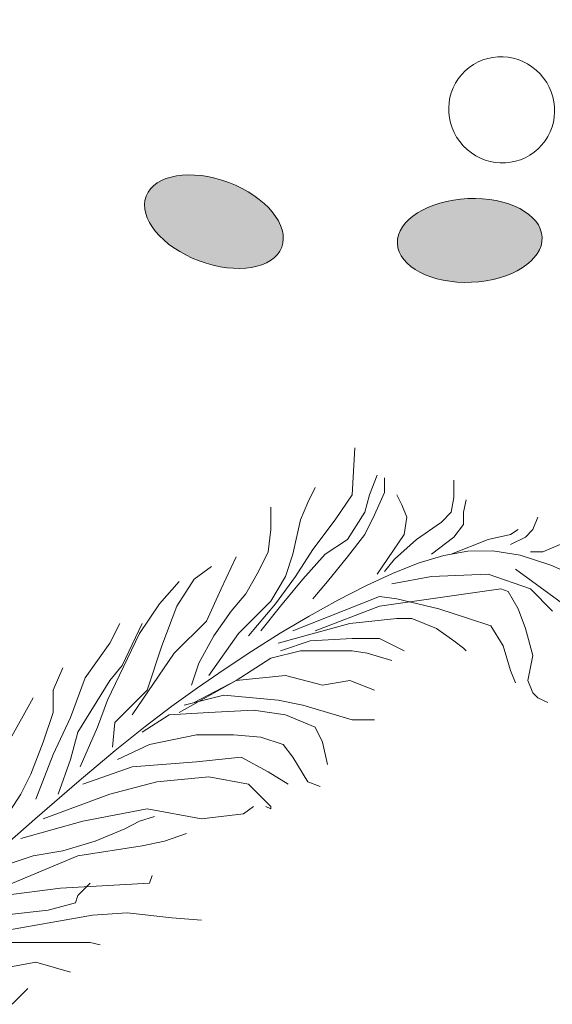
# Model space of a CAD drawing. Units: millimetres. Extents: x 595116 to 630915, y 909473 to 920225.
# Tile 103 of 134: x 629807.854 to 629812.676, y 919172.104 to 919181.018. Entities that reach past the tile are written whole.
import ezdxf

# ---------------------------------------------------------------- set-up
doc = ezdxf.new("R2010")
doc.units = ezdxf.units.MM
doc.layers.add('L-PLNT', color=85, linetype='Continuous', lineweight=13)

# ---------------------------------------------------------------- blocks, each defined once
blk = doc.blocks.new('A$C4FB75ABC')
for p, q in [((4.1608, 3.5609), (4.1668, 3.6742)), ((4.2026, 3.5609), (4.2205, 3.6086)), ((4.2384, 3.5668), (4.2384, 3.6026)), ((4.4054, 3.5549), (4.4054, 3.5967)), ((4.0535, 3.543), (4.0714, 3.5788)), ((4.2145, 3.5132), (4.2384, 3.5668)), ((4.0356, 3.5013), (4.0535, 3.543)), ((4.1191, 3.5013), (4.1608, 3.5609)), ((4.1907, 3.5192), (4.2026, 3.5609)), ((4.2801, 3.537), (4.2682, 3.5609)), ((4.3994, 3.5192), (4.4054, 3.5549)), ((4.4293, 3.5192), (4.4352, 3.549)), ((3.964, 3.4774), (3.964, 3.5311)), ((4.1489, 3.4536), (4.1907, 3.5192)), ((4.2921, 3.5072), (4.2801, 3.537)), ((4.3756, 3.4953), (4.3994, 3.5192)), ((4.4293, 3.4893), (4.4293, 3.5192)), ((4.0177, 3.4178), (4.0356, 3.5013)), ((4.0654, 3.4297), (4.1191, 3.5013)), ((4.1907, 3.4655), (4.2145, 3.5132)), ((4.2861, 3.4655), (4.2921, 3.5072)), ((4.3159, 3.4536), (4.3756, 3.4953)), ((4.5963, 3.4774), (4.6082, 3.5072)), ((3.958, 3.4238), (3.964, 3.4774)), ((4.4054, 3.4595), (4.4293, 3.4893)), ((4.5426, 3.4655), (4.5605, 3.4774)), ((4.5784, 3.4595), (4.5963, 3.4774)), ((4.0952, 3.4178), (4.1489, 3.4536)), ((4.1489, 3.4118), (4.1907, 3.4655)), ((4.2205, 3.3701), (4.2861, 3.4655)), ((4.2622, 3.4059), (4.3159, 3.4536)), ((4.3517, 3.4178), (4.4054, 3.4595)), ((4.3994, 3.4178), (4.4889, 3.4536)), ((4.4889, 3.4536), (4.5426, 3.4655)), ((4.5426, 3.4416), (4.5784, 3.4595)), ((3.9342, 3.3761), (3.958, 3.4238)), ((4.0237, 3.3641), (4.0654, 3.4297)), ((4.3813, 3.4152), (4.4396, 3.4254)), ((4.4396, 3.4254), (4.5001, 3.426)), ((4.5001, 3.426), (4.5657, 3.4153)), ((4.5903, 3.4238), (4.6201, 3.4238)), ((4.6201, 3.4238), (4.6619, 3.4416)), ((3.8447, 3.3343), (3.8805, 3.4118)), ((3.9998, 3.3641), (4.0177, 3.4178)), ((4.0415, 3.3582), (4.0952, 3.4178)), ((4.1012, 3.3522), (4.1489, 3.4118)), ((4.2384, 3.3761), (4.2622, 3.4059)), ((4.2593, 3.3722), (4.322, 3.3969)), ((4.322, 3.3969), (4.3813, 3.4152)), ((4.5657, 3.4153), (4.6395, 3.3917)), ((3.7791, 3.3582), (3.8208, 3.388)), ((3.9044, 3.3224), (3.9342, 3.3761)), ((4.1935, 3.342), (4.2593, 3.3722)), ((4.5545, 3.382), (4.6858, 3.2866)), ((4.6395, 3.3917), (4.7247, 3.3534)), ((3.6956, 3.2986), (3.7433, 3.3522)), ((3.7373, 3.2926), (3.7791, 3.3582)), ((3.964, 3.3045), (3.9998, 3.3641)), ((3.9759, 3.2986), (4.0237, 3.3641)), ((3.9879, 3.2926), (4.0415, 3.3582)), ((4.0654, 3.3105), (4.1012, 3.3522)), ((4.2563, 3.3463), (4.3517, 3.3641)), ((4.3517, 3.3641), (4.4889, 3.3701)), ((4.4889, 3.3701), (4.5903, 3.3343)), ((3.8089, 3.2568), (3.8447, 3.3343)), ((4.1256, 3.3072), (4.1935, 3.342)), ((4.2265, 3.2926), (4.5187, 3.3343)), ((4.5187, 3.3343), (4.5366, 3.3284)), ((4.5366, 3.3284), (4.5605, 3.2866)), ((4.5903, 3.3343), (4.644, 3.2807)), ((3.8686, 3.2807), (3.9044, 3.3224)), ((3.8865, 3.227), (3.964, 3.3045)), ((4.0177, 3.233), (4.2265, 3.3164)), ((4.0565, 3.2687), (4.1256, 3.3072)), ((4.2265, 3.3164), (4.2682, 3.3105)), ((4.2682, 3.3105), (4.3696, 3.2866)), ((3.6479, 3.227), (3.6956, 3.2986)), ((3.7015, 3.1972), (3.7373, 3.2926)), ((3.8268, 3.2211), (3.8686, 3.2807)), ((3.9103, 3.2211), (3.9759, 3.2986)), ((3.9401, 3.233), (3.9879, 3.2926)), ((4.0714, 3.233), (4.2265, 3.2926)), ((4.3696, 3.2866), (4.4412, 3.2628)), ((4.5605, 3.2866), (4.5784, 3.2389)), ((3.7314, 3.1793), (3.8089, 3.2568)), ((3.9871, 3.2274), (4.0565, 3.2687)), ((4.1549, 3.2509), (4.2682, 3.2628)), ((4.2682, 3.2628), (4.304, 3.2628)), ((4.304, 3.2628), (4.3637, 3.2389)), ((4.4412, 3.2628), (4.4949, 3.2449)), ((3.5763, 3.2032), (3.6001, 3.2509)), ((3.6061, 3.1495), (3.6538, 3.2509)), ((3.9819, 3.2032), (4.1549, 3.2509)), ((4.3637, 3.2389), (4.4054, 3.2091)), ((4.4949, 3.2449), (4.5247, 3.1972)), ((4.5784, 3.2389), (4.5963, 3.1734)), ((3.5703, 3.066), (3.6479, 3.227)), ((3.791, 3.1555), (3.8268, 3.2211)), ((3.8149, 3.1257), (3.8865, 3.227)), ((3.9185, 3.1843), (3.9871, 3.2274)), ((3.9879, 3.1853), (4.0594, 3.2091)), ((4.0594, 3.2091), (4.1608, 3.2151)), ((4.1608, 3.2151), (4.2265, 3.2151)), ((4.2265, 3.2151), (4.2861, 3.1853)), ((4.4054, 3.2091), (4.4293, 3.1912)), ((3.5166, 3.1197), (3.5763, 3.2032)), ((3.6658, 3.0899), (3.7015, 3.1972)), ((3.8516, 3.1401), (3.9185, 3.1843)), ((3.964, 3.1674), (4.0356, 3.1853)), ((4.0356, 3.1853), (4.1072, 3.1853)), ((4.1072, 3.1853), (4.1608, 3.1853)), ((4.1608, 3.1853), (4.1966, 3.1793)), ((4.4293, 3.1912), (4.4352, 3.1853)), ((4.5247, 3.1972), (4.5426, 3.1376)), ((3.63, 3.0303), (3.7314, 3.1793)), ((3.8805, 3.1137), (3.964, 3.1674)), ((4.1966, 3.1793), (4.2563, 3.1614)), ((4.5963, 3.1734), (4.5844, 3.1137)), ((3.4391, 3.0899), (3.4629, 3.1436)), ((3.5763, 3.1137), (3.6061, 3.1495)), ((3.7731, 3.1018), (3.791, 3.1555)), ((3.7873, 3.0958), (3.8516, 3.1401)), ((4.5426, 3.1376), (4.5545, 3.1078)), ((3.4808, 3.0243), (3.5166, 3.1197)), ((3.4987, 2.9885), (3.5763, 3.1137)), ((3.7433, 3.0362), (3.8805, 3.1137)), ((3.7791, 3.0601), (3.8805, 3.1137)), ((3.8805, 3.1137), (3.9998, 3.1257)), ((3.9998, 3.1257), (4.0893, 3.1018)), ((4.0893, 3.1018), (4.1549, 3.1137)), ((4.1549, 3.1137), (4.2145, 3.0899)), ((4.5844, 3.1137), (4.5963, 3.0839)), ((3.4391, 3.0362), (3.4391, 3.0899)), ((3.5882, 3.0124), (3.6658, 3.0899)), ((3.7254, 3.0513), (3.7873, 3.0958)), ((3.3317, 2.9647), (3.3914, 3.072)), ((3.5465, 3.0005), (3.5703, 3.066)), ((3.7552, 3.0541), (3.8507, 3.078)), ((3.8507, 3.078), (3.9819, 3.066)), ((3.9819, 3.066), (4.0415, 3.0541)), ((4.5963, 3.0839), (4.6082, 3.072)), ((4.6082, 3.072), (4.6321, 3.0601)), ((3.6611, 3.0024), (3.7254, 3.0513)), ((3.8149, 3.0362), (3.9222, 3.0422)), ((3.9222, 3.0422), (3.9998, 3.0303)), ((4.0415, 3.0541), (4.1608, 3.0184)), ((3.4152, 2.9647), (3.4391, 3.0362)), ((3.4391, 2.9349), (3.4808, 3.0243)), ((3.6538, 2.9885), (3.7194, 3.0303)), ((3.7194, 3.0303), (3.8149, 3.0362)), ((3.9998, 3.0303), (4.0714, 3.0005)), ((4.1608, 3.0184), (4.2145, 3.0184)), ((3.5047, 2.9051), (3.5465, 3.0005)), ((3.5822, 2.9528), (3.5882, 3.0124)), ((3.5886, 2.9442), (3.6611, 3.0024)), ((4.0714, 3.0005), (4.0893, 2.9647)), ((3.4808, 2.923), (3.4987, 2.9885)), ((3.6717, 2.9587), (3.7851, 2.9826)), ((3.7851, 2.9826), (3.8745, 2.9826)), ((3.8745, 2.9826), (3.9401, 2.9766)), ((3.9401, 2.9766), (3.9938, 2.9587)), ((3.3854, 2.8872), (3.4152, 2.9647)), ((3.5942, 2.923), (3.6717, 2.9587)), ((3.9938, 2.9587), (4.0177, 2.9289)), ((4.0893, 2.9647), (4.1012, 2.911)), ((3.3973, 2.8276), (3.4391, 2.9349)), ((3.451, 2.8395), (3.4808, 2.923)), ((3.5019, 2.8714), (3.5886, 2.9442)), ((3.7851, 2.917), (3.8924, 2.9289)), ((3.8924, 2.9289), (3.958, 2.8932)), ((4.0177, 2.9289), (4.0535, 2.8693)), ((3.5107, 2.8633), (3.63, 2.9051)), ((3.63, 2.9051), (3.7851, 2.917)), ((3.3615, 2.8395), (3.3854, 2.8872)), ((3.6896, 2.8693), (3.8149, 2.8812)), ((3.8149, 2.8812), (3.9103, 2.8633)), ((3.958, 2.8932), (4.0058, 2.8633)), ((3.3951, 2.779), (3.5019, 2.8714)), ((3.5763, 2.8395), (3.6896, 2.8693)), ((3.9103, 2.8633), (3.964, 2.8097)), ((4.0535, 2.8693), (4.0833, 2.8574)), ((3.2721, 2.7024), (3.3615, 2.8395)), ((3.4152, 2.7799), (3.5763, 2.8395)), ((3.5107, 2.7739), (3.6658, 2.8037)), ((3.6658, 2.8037), (3.797, 2.7799)), ((3.8984, 2.7918), (3.9222, 2.8097)), ((3.964, 2.8037), (3.9521, 2.8097)), ((3.964, 2.8097), (3.964, 2.8037)), ((3.2623, 2.6619), (3.3951, 2.779)), ((3.6479, 2.7739), (3.6837, 2.7858)), ((3.797, 2.7799), (3.8984, 2.7918)), ((3.3615, 2.7322), (3.5107, 2.7739)), ((3.5405, 2.7262), (3.6121, 2.756)), ((3.6121, 2.756), (3.6479, 2.7739)), ((3.7075, 2.7262), (3.7612, 2.7441)), ((3.4629, 2.7024), (3.5405, 2.7262)), ((3.4987, 2.6904), (3.6538, 2.7143)), ((3.6538, 2.7143), (3.7075, 2.7262)), ((3.2422, 2.5831), (3.4987, 2.6904)), ((3.284, 2.6547), (3.3914, 2.6904)), ((3.3914, 2.6904), (3.4629, 2.7024)), ((3.6717, 2.6249), (3.6777, 2.6428)), ((3.3198, 2.5951), (3.457, 2.6129)), ((3.457, 2.6129), (3.6717, 2.6249)), ((3.4987, 2.5951), (3.5286, 2.6249)), ((3.4928, 2.5772), (3.4987, 2.5951)), ((3.4272, 2.5593), (3.4928, 2.5772)), ((3.1289, 2.4758), (3.5345, 2.5474)), ((3.3198, 2.5474), (3.4272, 2.5593)), ((3.5345, 2.5474), (3.618, 2.5533)), ((3.618, 2.5533), (3.7254, 2.5414)), ((3.7254, 2.5414), (3.797, 2.5354)), ((3.3019, 2.4818), (3.4152, 2.4818)), ((3.4152, 2.4818), (3.5286, 2.4818)), ((3.5286, 2.4818), (3.5524, 2.4758)), ((3.3019, 2.4162), (3.3973, 2.4341)), ((3.3973, 2.4341), (3.4808, 2.4102)), ((3.3403, 2.3324), (3.3784, 2.3706))]:
    blk.add_line(p, q)
blk = doc.blocks.new('A$C77972600')
h = blk.add_hatch(color=256)
edge = h.paths.add_edge_path()
edge.add_ellipse((3.2403, 1.6985), major_axis=(-0.1668, -0.0838), ratio=0.578492, start_angle=0, end_angle=360, ccw=False)
edge = h.paths.add_edge_path()
edge.add_ellipse((4.2796, 1.6084), major_axis=(-0.1206, -0.1425), ratio=0.578492, start_angle=0, end_angle=360, ccw=False)
edge = h.paths.add_edge_path()
edge.add_ellipse((4.7739, 0.881), major_axis=(-0.1747, 0.0657), ratio=0.578492, start_angle=0, end_angle=360, ccw=False)
edge = h.paths.add_edge_path()
edge.add_ellipse((5.4333, 0.8328), major_axis=(-0.1865, -0.008), ratio=0.578492, start_angle=0, end_angle=360, ccw=False)
edge = h.paths.add_edge_path()
edge.add_ellipse((4.6573, 4.2045), major_axis=(-0.1865, -0.008), ratio=0.578492, start_angle=0, end_angle=360, ccw=False)
edge = h.paths.add_edge_path()
edge.add_ellipse((4.556, 3.4032), major_axis=(-0.1865, -0.008), ratio=0.578492, start_angle=0, end_angle=360, ccw=False)
edge = h.paths.add_edge_path()
edge.add_ellipse((4.9297, 3.677), major_axis=(-0.1668, -0.0838), ratio=0.578492, start_angle=0, end_angle=360, ccw=False)
edge = h.paths.add_edge_path()
edge.add_ellipse((3.7756, 2.5742), major_axis=(-0.1206, -0.1425), ratio=0.578492, start_angle=0, end_angle=360, ccw=False)
edge = h.paths.add_edge_path()
edge.add_ellipse((3.1788, 2.8466), major_axis=(-0.1206, -0.1425), ratio=0.578492, start_angle=0, end_angle=360, ccw=False)
edge = h.paths.add_edge_path()
edge.add_ellipse((3.8763, 3.0252), major_axis=(-0.1206, -0.1425), ratio=0.578492, start_angle=0, end_angle=360, ccw=False)
edge = h.paths.add_edge_path()
edge.add_ellipse((2.3609, 1.8217), major_axis=(-0.1865, -0.008), ratio=0.578492, start_angle=0, end_angle=360, ccw=False)
edge = h.paths.add_edge_path()
edge.add_ellipse((3.0627, 1.8578), major_axis=(-0.1865, -0.008), ratio=0.578492, start_angle=0, end_angle=360, ccw=False)
edge = h.paths.add_edge_path()
edge.add_ellipse((2.7605, 2.0535), major_axis=(-0.1865, -0.008), ratio=0.578492, start_angle=0, end_angle=360, ccw=False)
edge = h.paths.add_edge_path()
edge.add_ellipse((2.1439, 3.4246), major_axis=(-0.1668, -0.0838), ratio=0.578492, start_angle=0, end_angle=360, ccw=False)
edge = h.paths.add_edge_path()
edge.add_ellipse((4.2959, 2.0225), major_axis=(-0.1747, 0.0657), ratio=0.578492, start_angle=0, end_angle=360, ccw=False)
edge = h.paths.add_edge_path()
edge.add_ellipse((1.9127, 4.2528), major_axis=(-0.1865, -0.008), ratio=0.578492, start_angle=0, end_angle=360, ccw=False)
edge = h.paths.add_edge_path()
edge.add_ellipse((1.5555, 4.1052), major_axis=(-0.1747, 0.0657), ratio=0.578492, start_angle=0, end_angle=360, ccw=False)
edge = h.paths.add_edge_path()
edge.add_ellipse((0.9962, 4.2695), major_axis=(-0.1865, -0.008), ratio=0.578492, start_angle=0, end_angle=360, ccw=False)
edge = h.paths.add_edge_path()
edge.add_ellipse((1.2179, 3.5926), major_axis=(-0.1747, 0.0657), ratio=0.578492, start_angle=0, end_angle=360, ccw=False)
edge = h.paths.add_edge_path()
edge.add_ellipse((1.6764, 3.6493), major_axis=(-0.1747, 0.0657), ratio=0.578492, start_angle=0, end_angle=360, ccw=False)
edge = h.paths.add_edge_path()
edge.add_ellipse((0.8384, 2.8599), major_axis=(-0.1668, -0.0838), ratio=0.578492, start_angle=0, end_angle=360, ccw=False)
edge = h.paths.add_edge_path()
edge.add_ellipse((0.9659, 2.049), major_axis=(-0.1206, -0.1425), ratio=0.578492, start_angle=0, end_angle=360, ccw=False)
edge = h.paths.add_edge_path()
edge.add_ellipse((1.3147, 2.1383), major_axis=(-0.1206, -0.1425), ratio=0.578492, start_angle=0, end_angle=360, ccw=False)
edge = h.paths.add_edge_path()
edge.add_ellipse((5.4586, 2.9929), major_axis=(-0.1865, -0.008), ratio=0.578492, start_angle=0, end_angle=360, ccw=False)
edge = h.paths.add_edge_path()
edge.add_ellipse((3.4224, 5.3915), major_axis=(-0.1865, -0.008), ratio=0.578492, start_angle=0, end_angle=360, ccw=False)
edge = h.paths.add_edge_path()
edge.add_ellipse((3.7245, 5.1958), major_axis=(-0.1865, -0.008), ratio=0.578492, start_angle=0, end_angle=360, ccw=False)
edge = h.paths.add_edge_path()
edge.add_ellipse((4.5588, 5.4431), major_axis=(-0.1668, -0.0838), ratio=0.578492, start_angle=0, end_angle=360, ccw=False)
edge = h.paths.add_edge_path()
edge.add_ellipse((4.4393, 4.7252), major_axis=(-0.1668, -0.0838), ratio=0.578492, start_angle=0, end_angle=360, ccw=False)
edge = h.paths.add_edge_path()
edge.add_ellipse((4.7087, 5.1006), major_axis=(-0.1668, -0.0838), ratio=0.578492, start_angle=0, end_angle=360, ccw=False)
edge = h.paths.add_edge_path()
edge.add_ellipse((3.7138, 4.6852), major_axis=(-0.1668, -0.0838), ratio=0.578492, start_angle=0, end_angle=360, ccw=False)
blk.add_ellipse((5.5155, 1.1693), major_axis=(-0.0941, 0.1005), ratio=0.985729)
at = {"extrusion": (0, 0, -1)}
blk.add_ellipse((4.7739, 0.881), major_axis=(-0.1747, 0.0657), ratio=0.578492, dxfattribs=at)
blk.add_ellipse((5.4333, 0.8328), major_axis=(-0.1865, -0.008), ratio=0.578492, start_param=3.141593, end_param=9.424778, dxfattribs=at)

msp = doc.modelspace()

# ---------------------------------------------------------------- block references
at = {"layer": 'L-PLNT'}
for name, p, xscale, yscale, zscale in [('A$C77972600', (629792.8437, 919176.0945), 3.512546757812034, 3.512546757812034, 3.512546757812034), ('A$C4FB75ABC', (629795.2477, 919163.3497), 3.753413438031968, 3.753413438031968, 3.753413438031968)]:
    msp.add_blockref(name, p, dxfattribs=dict(at, xscale=xscale, yscale=yscale, zscale=zscale))

doc.saveas('drawing.dxf')
